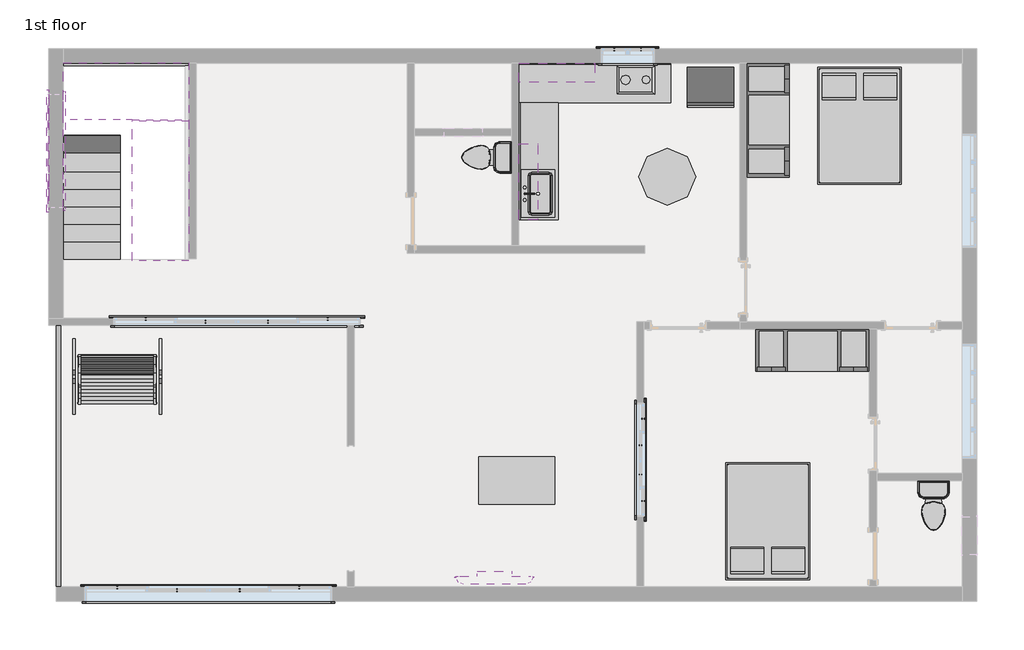
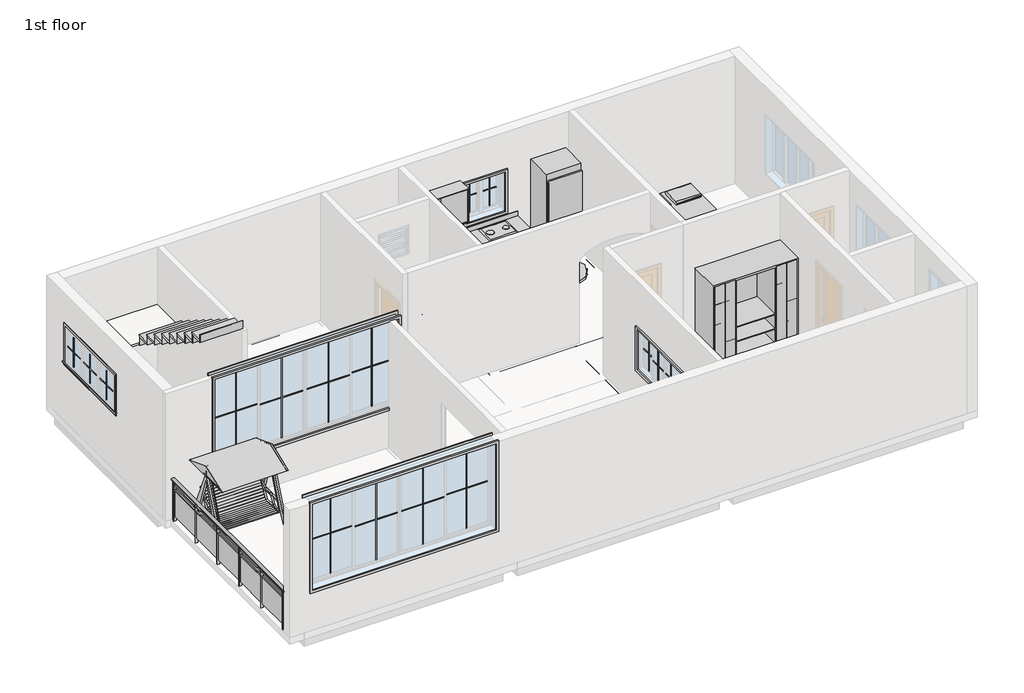
# One storey, part 2 of 2: 30 proxies, 16 furniture elements, 8 beams, 3 flow terminals, 2 stair flights, 1 railing, 1 slab.
# Revit data of these elements (continued)
# Materials (continued)
#   "Laminate, Linen, Matte": class "Plastic", colour RGB 249 239 230, transparency 0, Description = "Plastic Laminate - Linen, Matte", Cost = 0
#   "Wood - Birch": class "Wood", colour RGB 224 178 126, transparency 0
#   "Laminate - Ivory, Matte": colour RGB 247 247 239, transparency 0
#   "Cabinets": colour RGB 249 249 249, transparency 0
#   "Cabinets - Handles": colour RGB 57 57 57, transparency 0
#   "Birch": class "Wood", colour RGB 224 178 126, transparency 0, Description = "Betula Alleghaniensis", Cost = 0
#   "Linen, White": class "Textile", colour RGB 247 247 239, transparency 0, Description = "Linen, white", Cost = 0
#   "Glass - Clear, Grey": class "Glass", colour RGB 252 255 255, transparency 0.64
#   "Pine": class "Wood", colour RGB 223 192 134, transparency 0, Description = "Pinus Echinata", Cost = 0
#   "Clad - White": class "Wood", colour RGB 242 242 238, transparency 0, Cost = 0
#   "Wood - Stained": class "Wood", colour RGB 224 178 126, transparency 0, Cost = 0
#   "wood finish": class "Generic", colour RGB 120 120 120, transparency 0, Cost = 0
#   "steel": class "Generic", colour RGB 120 120 120, transparency 0, Cost = 0
#   "fabric": class "Generic", colour RGB 120 120 120, transparency 0, Cost = 0
#   "Cabinet": colour RGB 204 122 2, transparency 0
#   "Counter Top": class "Wood", colour RGB 226 177 128, transparency 0
#   "Steel, Chrome Plated": class "Metal", colour RGB 17 17 17, transparency 0, Description = "Chromiuim plated steel", Cost = 0
#   "TV - Black": colour RGB 49 49 49, transparency 0
#   "TV - Glass": colour RGB 157 157 157, transparency 0.9
#   "TV - Screen": colour RGB 0 0 0, transparency 0
#   "Glass": class "Glass", colour RGB 0 128 192, transparency 0.75, Description = "Soda Lime Glass", Cost = 0
